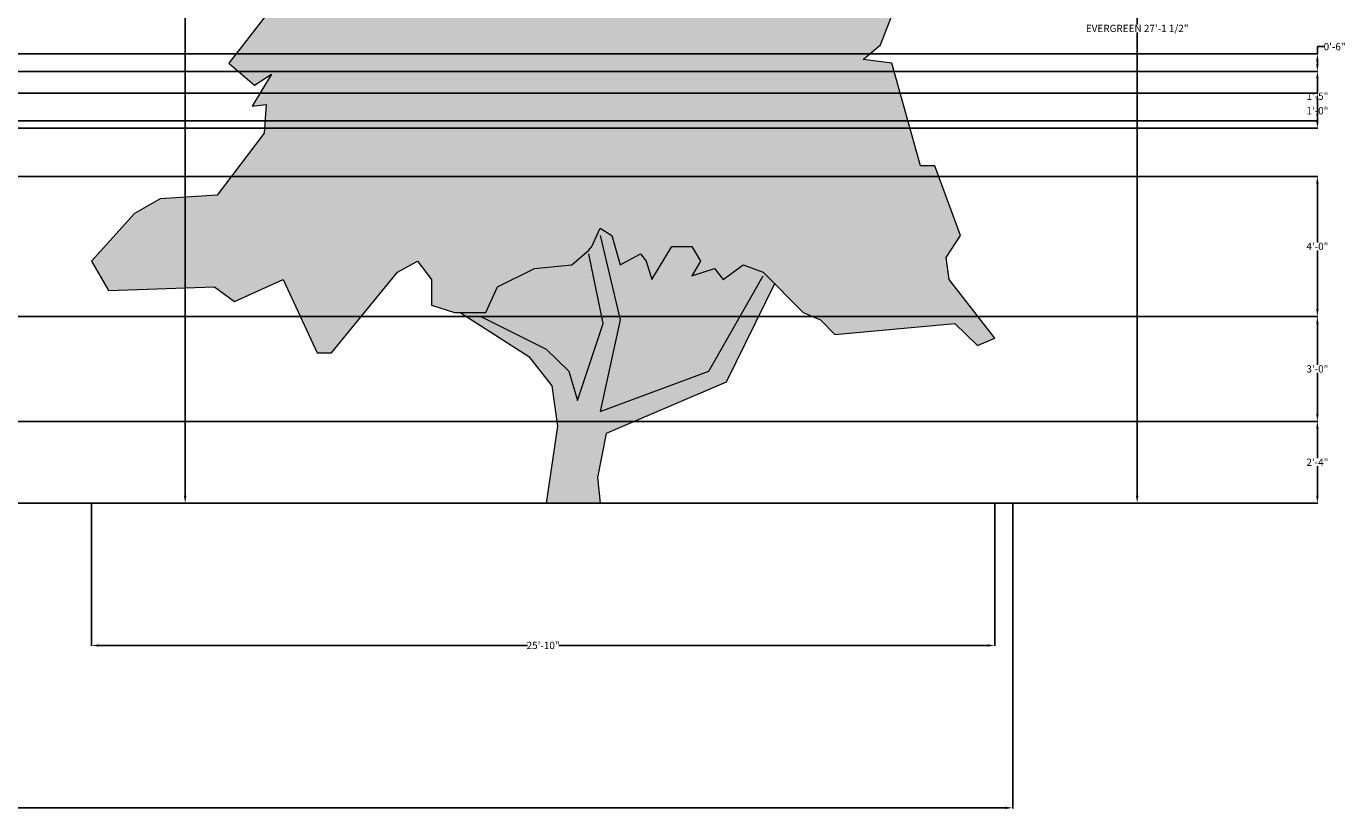
# Model space of a CAD drawing. Units: inches. Extents: x 481 to 2783, y 1975 to 3327.
# Tile 12 of 13: x 2331 to 2783, y 2017 to 2286. Entities that reach past the tile are written whole.
import ezdxf

# ---------------------------------------------------------------- set-up
doc = ezdxf.new("R2010")
doc.units = ezdxf.units.IN
doc.header["$MEASUREMENT"] = 0
for name, color, linetype, lineweight in [('A-ANNO-DIMS', 50, 'Continuous', 18), ('C-TOPO', 7, 'Continuous', 25), ('L-PLNT', 7, 'Continuous', 13)]:
    doc.layers.add(name, color=color, linetype=linetype, lineweight=lineweight)
doc.layers.add('L-PLNT-PATT', color=116, linetype='Continuous', lineweight=13, true_color=0x136734)
doc.layers.add('L-PLNT-TRNK-PATT', color=249, linetype='Continuous', lineweight=13, true_color=0x593132)
doc.styles.get("Standard").update_dxf_attribs({"font": 'arial.ttf'})
doc.dimstyles.get("Standard").update_dxf_attribs({"dimtxt": 2.5, "dimasz": 2.5, "dimexe": 0.18, "dimexo": 0.0625, "dimgap": 0.09, "dimtad": 0, "dimtih": 1, "dimtoh": 1, "dimzin": 0, "dimdsep": 46, "dimlunit": 3, "dimtxsty": 'Standard', "dimcen": 0.09, "dimadec": 0, "dimazin": 0, "dimtfac": 1, "dimtofl": 0, "dimtmove": 0, "dimatfit": 3, "dimfxl": 1, "dimtolj": 1, "dimtzin": 0, "dimarcsym": 0})

# ---------------------------------------------------------------- blocks, each defined once
blk = doc.blocks.new('Tree - type 3 evergreen elevation')
for points in [[(22.0124, 137.721), (18.5475, 141.5624), (15.5282, 138.2446), (13.8028, 139.3505), (13.3714, 142.1153), (11.2148, 143.2214), (8.1954, 140.4564), (4.7447, 141.0094), (2.1567, 136.0326), (2.1567, 131.6088), (5.6074, 129.9499), (3.0193, 128.2909), (0.4313, 130.5029), (-6.9015, 123.3141), (-6.9015, 121.6552), (-9.9208, 119.9963), (-9.0581, 118.3373), (-6.9015, 115.0195), (-10.7835, 112.2546), (-14.6656, 115.0195), (-16.8222, 114.4665), (-17.6849, 112.2546), (-14.6656, 111.7016), (-14.2342, 107.2778), (-17.6065, 107.8307), (-21.5669, 103.9599), (-17.2536, 103.4069), (-18.9789, 97.8771), (-22.8609, 97.3241), (-27.1743, 94.5593), (-32.3504, 91.7944), (-32.7817, 94.0063), (-36.6638, 85.7116), (-29.7624, 87.3705), (-25.449, 84.6056), (-26.743, 77.9699), (-34.507, 75.205), (-37.9578, 77.4169), (-39.2518, 74.099), (-42.2711, 73.5461), (-44.8592, 70.2282), (-47.8786, 66.3574), (-43.9965, 63.0395), (-41.4085, 64.6985), (-44.3346, 59.8898), (-42.2089, 60.1377), (-42.5159, 55.7849), (-49.6039, 46.4502), (-58.2307, 45.8972), (-62.1127, 43.6853), (-68.5828, 36.4966), (-65.9947, 32.0727), (-50.0352, 32.6257), (-47.0159, 30.4138), (-39.6831, 33.7317), (-34.507, 22.6721), (-32.3504, 22.6721), (-22.4296, 34.8376), (-19.4102, 36.4966), (-17.2536, 33.7317), (-17.2536, 29.8608), (-13.8028, 28.7549), (-9.0581, 28.7549), (-7.3328, 32.6257), (-1.7254, 35.3906), (3.8821, 35.9436), (6.4701, 38.1555), (6.9014, 38.7085), (8.1954, 41.4734), (9.9208, 40.3674), (11.2148, 35.9436), (14.2341, 37.6025), (15.0968, 36.4966), (15.9595, 33.7317), (18.9789, 38.7085), (21.9982, 38.7085), (23.2922, 36.4966), (21.9982, 34.2847), (25.4489, 35.3906), (26.743, 33.7317), (29.7623, 35.9436), (32.7817, 34.8376), (38.8204, 28.7549), (41.4084, 27.6489), (43.5651, 25.437), (61.6813, 27.0959), (65.132, 23.7781), (67.7201, 24.884), (60.8186, 33.7317), (60.3873, 37.0495), (62.544, 40.3674), (58.662, 50.874), (56.5053, 50.874), (52.1919, 66.3574), (47.8785, 66.9103), (50.4665, 69.1222), (53.9172, 77.9699), (47.0158, 85.1586), (38.3891, 87.9235), (42.2711, 94.0063)], [(42.2711, 94.0063), (38.8204, 104.5129), (36.6637, 104.5129), (32.3503, 113.9135), (29.7623, 113.3605), (26.743, 113.3605), (24.5862, 117.7844), (25.8802, 123.8671), (29.331, 123.8671), (22.8609, 131.6088), (21.9982, 137.6916)], [(8.1954, 40.3674), (11.2148, 27.6489), (8.1954, 13.8245), (24.5862, 19.9072), (32.7817, 34.2847)], [(-9.9208, 28.2019), (0, 23.2251), (3.4507, 19.9072), (4.7447, 15.4834), (8.6267, 27.0959), (6.4701, 37.6025)], [(34.5071, 33.1787), (27.1743, 18.2483), (9.0581, 10.5066), (7.7641, 3.8708), (8.1954, 0)], [(-12.9401, 28.7549), (-2.588, 22.1191), (0.8626, 17.6953), (1.7253, 11.6125), (0, 0)]]:
    blk.add_lwpolyline(points)
blk = doc.blocks.new('*D56')
at = {"layer": 'A-ANNO-DIMS', "color": 0, "lineweight": -2, "transparency": 16777216}
for p, q in [((2321.97, 2546.55), (2385.65, 2546.55)), ((2385.47, 2544.05), (2385.47, 2336.07)), ((2385.47, 2125.32), (2385.47, 2333.3)), ((2321.97, 2122.82), (2385.65, 2122.82))]:
    blk.add_line(p, q, dxfattribs=at)
at = {"layer": 'A-ANNO-DIMS', "color": 0, "transparency": 16777216}
for points in [[(2385.05, 2544.05), (2385.89, 2544.05), (2385.47, 2546.55)], [(2385.05, 2125.32), (2385.89, 2125.32), (2385.47, 2122.82)]]:
    blk.add_solid(points, dxfattribs=at)
at = {"layer": 'Defpoints', "color": 0, "transparency": 16777216}
for p in [(2321.91, 2546.55), (2385.47, 2546.55), (2321.91, 2122.82)]:
    blk.add_point(p, dxfattribs=at)
at = {"layer": 'A-ANNO-DIMS', "color": 0, "transparency": 16777216, "insert": (2385.47, 2334.69), "char_height": 2.5, "attachment_point": 5}
blk.add_mtext('\\A1;PALM 35\'-3 1/2"', dxfattribs=at)
blk = doc.blocks.new('*D60')
at = {"layer": 'A-ANNO-DIMS', "color": 0, "lineweight": -2, "transparency": 16777216}
for p, q in [((2663.19, 2448.32), (2712.14, 2448.32)), ((2711.96, 2445.82), (2711.96, 2286.95)), ((2711.96, 2125.32), (2711.96, 2284.19)), ((2663.19, 2122.82), (2712.14, 2122.82))]:
    blk.add_line(p, q, dxfattribs=at)
at = {"layer": 'A-ANNO-DIMS', "color": 0, "transparency": 16777216}
for points in [[(2711.54, 2445.82), (2712.37, 2445.82), (2711.96, 2448.32)], [(2711.54, 2125.32), (2712.37, 2125.32), (2711.96, 2122.82)]]:
    blk.add_solid(points, dxfattribs=at)
at = {"layer": 'Defpoints', "color": 0, "transparency": 16777216}
for p in [(2663.13, 2448.32), (2711.96, 2448.32), (2663.13, 2122.82)]:
    blk.add_point(p, dxfattribs=at)
at = {"layer": 'A-ANNO-DIMS', "color": 0, "transparency": 16777216, "insert": (2711.96, 2285.57), "char_height": 2.5, "attachment_point": 5}
blk.add_mtext('\\A1;EVERGREEN 27\'-1 1/2"', dxfattribs=at)
blk = doc.blocks.new('*D61')
at = {"layer": 'A-ANNO-DIMS', "color": 0, "lineweight": -2, "transparency": 16777216}
for p, q in [((2353.35, 2122.76), (2353.35, 2073.82)), ((2663.13, 2122.76), (2663.13, 2073.82)), ((2355.85, 2074), (2502.87, 2074)), ((2660.63, 2074), (2513.62, 2074))]:
    blk.add_line(p, q, dxfattribs=at)
at = {"layer": 'A-ANNO-DIMS', "color": 0, "transparency": 16777216}
for points in [[(2355.85, 2074.41), (2355.85, 2073.58), (2353.35, 2074)], [(2660.63, 2074.41), (2660.63, 2073.58), (2663.13, 2074)]]:
    blk.add_solid(points, dxfattribs=at)
at = {"layer": 'Defpoints', "color": 0, "transparency": 16777216}
for p in [(2353.35, 2122.82), (2663.13, 2122.82), (2663.13, 2074)]:
    blk.add_point(p, dxfattribs=at)
at = {"layer": 'A-ANNO-DIMS', "color": 0, "transparency": 16777216, "insert": (2508.24, 2074), "char_height": 2.5, "attachment_point": 5}
blk.add_mtext('\\A1;25\'-10"', dxfattribs=at)
blk = doc.blocks.new('*D66')
at = {"layer": 'A-ANNO-DIMS', "color": 0, "lineweight": -2, "transparency": 16777216}
for p, q in [((591.06, 2122.76), (591.06, 2018.14)), ((2669.26, 2122.76), (2669.26, 2018.14)), ((593.56, 2018.32), (1624.92, 2018.32)), ((2666.76, 2018.32), (1635.4, 2018.32))]:
    blk.add_line(p, q, dxfattribs=at)
at = {"layer": 'A-ANNO-DIMS', "color": 0, "transparency": 16777216}
for points in [[(593.56, 2018.74), (593.56, 2017.9), (591.06, 2018.32)], [(2666.76, 2018.74), (2666.76, 2017.9), (2669.26, 2018.32)]]:
    blk.add_solid(points, dxfattribs=at)
at = {"layer": 'Defpoints', "color": 0, "transparency": 16777216}
for p in [(591.06, 2122.82), (2669.26, 2122.82), (2669.26, 2018.32)]:
    blk.add_point(p, dxfattribs=at)
at = {"layer": 'A-ANNO-DIMS', "color": 0, "transparency": 16777216, "insert": (1630.16, 2018.32), "char_height": 2.5, "attachment_point": 5}
blk.add_mtext('\\A1;173\'-2"', dxfattribs=at)
blk = doc.blocks.new('*D70')
at = {"layer": 'A-ANNO-DIMS', "color": 0, "lineweight": -2, "transparency": 16777216}
for p, q in [((1794.5, 2150.82), (2773.94, 2150.82)), ((2773.76, 2148.32), (2773.76, 2138.17)), ((2773.76, 2125.32), (2773.76, 2135.48)), ((1794.5, 2122.82), (2773.94, 2122.82))]:
    blk.add_line(p, q, dxfattribs=at)
at = {"layer": 'A-ANNO-DIMS', "color": 0, "transparency": 16777216}
for points in [[(2773.34, 2148.32), (2774.17, 2148.32), (2773.76, 2150.82)], [(2773.34, 2125.32), (2774.17, 2125.32), (2773.76, 2122.82)]]:
    blk.add_solid(points, dxfattribs=at)
at = {"layer": 'Defpoints', "color": 0, "transparency": 16777216}
for p in [(1794.44, 2150.82), (2773.76, 2150.82), (1794.44, 2122.82)]:
    blk.add_point(p, dxfattribs=at)
at = {"layer": 'A-ANNO-DIMS', "color": 0, "transparency": 16777216, "insert": (2773.76, 2136.82), "char_height": 2.5, "attachment_point": 5}
blk.add_mtext('\\A1;2\'-4"', dxfattribs=at)
blk = doc.blocks.new('*D71')
at = {"layer": 'A-ANNO-DIMS', "color": 0, "lineweight": -2, "transparency": 16777216}
for p, q in [((1737.9, 2186.82), (2773.94, 2186.82)), ((2773.76, 2184.32), (2773.76, 2170.19)), ((2773.76, 2153.32), (2773.76, 2167.45)), ((1794.5, 2150.82), (2773.94, 2150.82))]:
    blk.add_line(p, q, dxfattribs=at)
at = {"layer": 'A-ANNO-DIMS', "color": 0, "transparency": 16777216}
for points in [[(2773.34, 2184.32), (2774.17, 2184.32), (2773.76, 2186.82)], [(2773.34, 2153.32), (2774.17, 2153.32), (2773.76, 2150.82)]]:
    blk.add_solid(points, dxfattribs=at)
at = {"layer": 'Defpoints', "color": 0, "transparency": 16777216}
for p in [(1737.84, 2186.82), (2773.76, 2186.82), (1794.44, 2150.82)]:
    blk.add_point(p, dxfattribs=at)
at = {"layer": 'A-ANNO-DIMS', "color": 0, "transparency": 16777216, "insert": (2773.76, 2168.82), "char_height": 2.5, "attachment_point": 5}
blk.add_mtext('\\A1;3\'-0"', dxfattribs=at)
blk = doc.blocks.new('*D72')
at = {"layer": 'A-ANNO-DIMS', "color": 0, "lineweight": -2, "transparency": 16777216}
for p, q in [((1737.9, 2234.82), (2773.94, 2234.82)), ((2773.76, 2232.32), (2773.76, 2212.19)), ((2773.76, 2189.32), (2773.76, 2209.45)), ((1737.9, 2186.82), (2773.94, 2186.82))]:
    blk.add_line(p, q, dxfattribs=at)
at = {"layer": 'A-ANNO-DIMS', "color": 0, "transparency": 16777216}
for points in [[(2773.34, 2232.32), (2774.17, 2232.32), (2773.76, 2234.82)], [(2773.34, 2189.32), (2774.17, 2189.32), (2773.76, 2186.82)]]:
    blk.add_solid(points, dxfattribs=at)
at = {"layer": 'Defpoints', "color": 0, "transparency": 16777216}
for p in [(1737.84, 2234.82), (2773.76, 2234.82), (1737.84, 2186.82)]:
    blk.add_point(p, dxfattribs=at)
at = {"layer": 'A-ANNO-DIMS', "color": 0, "transparency": 16777216, "insert": (2773.76, 2210.82), "char_height": 2.5, "attachment_point": 5}
blk.add_mtext('\\A1;4\'-0"', dxfattribs=at)
blk = doc.blocks.new('*D74')
at = {"layer": 'A-ANNO-DIMS', "color": 0, "lineweight": -2, "transparency": 16777216}
for p, q in [((1412.86, 2270.82), (2773.94, 2270.82)), ((2773.76, 2268.32), (2773.76, 2263.69)), ((2773.76, 2256.32), (2773.76, 2260.95)), ((1417, 2253.82), (2773.94, 2253.82))]:
    blk.add_line(p, q, dxfattribs=at)
at = {"layer": 'A-ANNO-DIMS', "color": 0, "transparency": 16777216}
for points in [[(2773.34, 2268.32), (2774.17, 2268.32), (2773.76, 2270.82)], [(2773.34, 2256.32), (2774.17, 2256.32), (2773.76, 2253.82)]]:
    blk.add_solid(points, dxfattribs=at)
at = {"layer": 'Defpoints', "color": 0, "transparency": 16777216}
for p in [(1412.79, 2270.82), (2773.76, 2270.82), (1416.94, 2253.82)]:
    blk.add_point(p, dxfattribs=at)
at = {"layer": 'A-ANNO-DIMS', "color": 0, "transparency": 16777216, "insert": (2773.76, 2262.32), "char_height": 2.5, "attachment_point": 5}
blk.add_mtext('\\A1;1\'-5"', dxfattribs=at)
blk = doc.blocks.new('*D75')
at = {"layer": 'A-ANNO-DIMS', "color": 0, "lineweight": -2, "transparency": 16777216}
for p, q in [((1794.5, 2276.82), (2773.94, 2276.82)), ((2773.76, 2276.82), (2773.76, 2279.32)), ((2773.76, 2279.32), (2776.26, 2279.32)), ((2773.76, 2273.32), (2773.76, 2274.32)), ((1794.5, 2270.82), (2773.94, 2270.82))]:
    blk.add_line(p, q, dxfattribs=at)
at = {"layer": 'A-ANNO-DIMS', "color": 0, "transparency": 16777216}
for points in [[(2773.34, 2274.32), (2774.17, 2274.32), (2773.76, 2276.82)], [(2773.34, 2273.32), (2774.17, 2273.32), (2773.76, 2270.82)]]:
    blk.add_solid(points, dxfattribs=at)
at = {"layer": 'Defpoints', "color": 0, "transparency": 16777216}
for p in [(1794.44, 2276.82), (2773.76, 2276.82), (1794.44, 2270.82)]:
    blk.add_point(p, dxfattribs=at)
at = {"layer": 'A-ANNO-DIMS', "color": 0, "transparency": 16777216, "insert": (2779.67, 2279.32), "char_height": 2.5, "attachment_point": 5}
blk.add_mtext('\\A1;0\'-6"', dxfattribs=at)
blk = doc.blocks.new('*D82')
at = {"layer": 'A-ANNO-DIMS', "color": 0, "lineweight": -2, "transparency": 16777216}
for p, q in [((1785.5, 2263.36), (2773.94, 2263.36)), ((2773.76, 2260.86), (2773.76, 2258.72)), ((2773.76, 2253.86), (2773.76, 2255.99)), ((1785.5, 2251.36), (2773.94, 2251.36))]:
    blk.add_line(p, q, dxfattribs=at)
at = {"layer": 'A-ANNO-DIMS', "color": 0, "transparency": 16777216}
for points in [[(2773.34, 2260.86), (2774.17, 2260.86), (2773.76, 2263.36)], [(2773.34, 2253.86), (2774.17, 2253.86), (2773.76, 2251.36)]]:
    blk.add_solid(points, dxfattribs=at)
at = {"layer": 'Defpoints', "color": 0, "transparency": 16777216}
for p in [(1785.44, 2263.36), (1785.44, 2251.36), (2773.76, 2251.36)]:
    blk.add_point(p, dxfattribs=at)
at = {"layer": 'A-ANNO-DIMS', "color": 0, "transparency": 16777216, "insert": (2773.76, 2257.36), "char_height": 2.5, "attachment_point": 5}
blk.add_mtext('\\A1;1\'-0"', dxfattribs=at)

msp = doc.modelspace()

# ---------------------------------------------------------------- hatches: boundary and pattern name
at = {"layer": 'L-PLNT-PATT'}
msp.add_hatch(color=256, dxfattribs=at).paths.add_polyline_path([(2476.873, 2366.633), (2469.209, 2367.89), (2460.208, 2359.093), (2470.011, 2357.836), (2466.089, 2345.268), (2457.267, 2344.011), (2447.464, 2337.728), (2435.7, 2331.444), (2434.72, 2336.471), (2425.897, 2317.619), (2441.582, 2321.389), (2451.385, 2315.106), (2448.444, 2300.025), (2430.798, 2293.741), (2422.956, 2298.768), (2420.015, 2291.227), (2413.153, 2289.97), (2407.271, 2282.43), (2400.408, 2273.633), (2409.231, 2266.092), (2415.113, 2269.862), (2408.463, 2258.933), (2413.294, 2259.497), (2412.596, 2249.604), (2396.487, 2228.389), (2376.881, 2227.132), (2368.058, 2222.105), (2353.354, 2205.767), (2359.236, 2195.713), (2395.507, 2196.97), (2402.369, 2191.943), (2419.035, 2199.483), (2430.798, 2174.348), (2435.7, 2174.348), (2458.247, 2201.997), (2465.109, 2205.767), (2470.011, 2199.483), (2470.011, 2190.686), (2477.853, 2188.172), (2488.637, 2188.172), (2492.558, 2196.97), (2505.302, 2203.254), (2518.046, 2204.51), (2523.928, 2209.537), (2524.908, 2210.794), (2527.849, 2217.078), (2531.77, 2214.564), (2534.711, 2204.51), (2541.573, 2208.281), (2543.534, 2205.767), (2545.495, 2199.483), (2552.357, 2210.794), (2559.219, 2210.794), (2562.16, 2205.767), (2559.219, 2200.74), (2567.062, 2203.254), (2570.003, 2199.483), (2576.865, 2204.51), (2583.727, 2201.997), (2597.451, 2188.172), (2603.333, 2185.659), (2608.235, 2180.632), (2649.408, 2184.402), (2657.25, 2176.862), (2663.132, 2179.375), (2647.447, 2199.483), (2646.467, 2207.024), (2651.368, 2214.564), (2642.546, 2238.443), (2637.644, 2238.443), (2627.841, 2273.633), (2618.038, 2274.889), (2623.92, 2279.916), (2631.762, 2300.025), (2616.077, 2316.362), (2596.471, 2322.646), (2605.294, 2336.471), (2597.451, 2360.349), (2592.55, 2360.349), (2582.746, 2381.714), (2576.865, 2380.458), (2570.003, 2380.458), (2565.101, 2390.512), (2568.042, 2404.336), (2575.884, 2404.336), (2561.18, 2421.931), (2559.202, 2435.877), (2551.377, 2444.553), (2544.515, 2437.012), (2540.593, 2439.526), (2539.613, 2445.809), (2534.711, 2448.323), (2527.849, 2442.039), (2520.007, 2443.296), (2514.125, 2431.985), (2514.125, 2421.931), (2521.967, 2418.161), (2516.085, 2414.39), (2510.203, 2419.417), (2493.538, 2403.079), (2493.538, 2399.309), (2486.676, 2395.539), (2488.637, 2391.768), (2493.538, 2384.228), (2484.715, 2377.944), (2475.892, 2384.228), (2470.991, 2382.971), (2469.03, 2377.944), (2475.892, 2376.687)])
at = {"layer": 'L-PLNT-TRNK-PATT'}
h = msp.add_hatch(color=256, dxfattribs=at)
h.paths.add_polyline_path([(2529.81, 2146.699), (2570.983, 2164.294), (2587.589, 2198.106), (2583.727, 2201.997), (2576.865, 2204.51), (2570.003, 2199.483), (2567.062, 2203.254), (2559.219, 2200.74), (2562.16, 2205.767), (2559.219, 2210.794), (2552.357, 2210.794), (2545.495, 2199.483), (2543.534, 2205.767), (2541.573, 2208.281), (2534.711, 2204.51), (2531.77, 2214.564), (2527.849, 2217.078), (2524.908, 2210.794), (2523.928, 2209.537), (2518.046, 2204.51), (2505.302, 2203.254), (2492.558, 2196.97), (2488.637, 2188.172), (2479.814, 2188.172), (2503.341, 2173.091), (2511.184, 2163.037), (2513.144, 2149.213), (2509.223, 2122.821), (2527.849, 2122.821), (2526.869, 2131.618)])
h.paths.add_polyline_path([(834.542, 2189.801), (831.106, 2193.262), (825, 2195.498), (818.895, 2191.026), (816.279, 2194.38), (809.302, 2192.144), (811.918, 2196.616), (809.302, 2201.089), (803.197, 2201.089), (797.091, 2191.026), (795.347, 2196.616), (793.603, 2198.852), (787.498, 2195.498), (784.881, 2204.443), (781.392, 2206.679), (778.776, 2201.089), (777.904, 2199.971), (772.671, 2195.498), (761.333, 2194.38), (749.995, 2188.789), (746.506, 2180.963), (738.657, 2180.963), (759.589, 2167.545), (766.566, 2158.6), (768.31, 2146.301), (764.821, 2122.821), (781.392, 2122.821), (780.52, 2130.647), (783.137, 2144.065), (819.768, 2159.718)])

# ---------------------------------------------------------------- linework, layer by layer
at = {"layer": 'C-TOPO'}
msp.add_line((1794.438, 2122.821), (2669.257, 2122.821), dxfattribs=at)

# ---------------------------------------------------------------- block references
at = {"layer": 'L-PLNT', "xscale": 2.272722171462171, "yscale": 2.272722171462171, "zscale": 2.272722171462171}
msp.add_blockref('Tree - type 3 evergreen elevation', (2509.223, 2122.821), dxfattribs=at)

# ---------------------------------------------------------------- dimensions: what is measured, and where the dimension line sits
at = {"layer": 'A-ANNO-DIMS'}
for base, p1, p2, text, picture, middle in [((2385.469, 2546.553), (2321.909, 2122.821), (2321.909, 2546.553), 'PALM <>', '*D56', (2385.469, 2334.687)), ((2711.958, 2448.323), (2663.132, 2122.821), (2663.132, 2448.323), 'EVERGREEN <>', '*D60', (2711.958, 2285.572))]:
    dim = msp.add_linear_dim(base=base, p1=p1, p2=p2, angle=90, text=text, dimstyle='Standard', override={"dimdec": 1, "dimlfac": 1, "dimrnd": 0, "dimzin": 1, "dimdsep": 46, "dimlunit": 4, "dimfrac": 2}, dxfattribs=at)
    dim.commit()
    dim.dimension.update_dxf_attribs({"geometry": picture, "text_midpoint": middle})
for base, p1, p2, picture, middle in [((2773.757, 2276.821), (1794.438, 2270.821), (1794.438, 2276.821), '*D75', (2779.67, 2279.321)), ((2773.757, 2270.821), (1416.938, 2253.821), (1412.793, 2270.821), '*D74', (2773.757, 2262.321)), ((2773.757, 2251.356), (1785.438, 2263.356), (1785.438, 2251.356), '*D82', (2773.757, 2257.356)), ((2773.757, 2234.821), (1737.842, 2186.821), (1737.842, 2234.821), '*D72', (2773.757, 2210.821)), ((2773.757, 2186.821), (1794.438, 2150.821), (1737.842, 2186.821), '*D71', (2773.757, 2168.821)), ((2773.757, 2150.821), (1794.438, 2122.821), (1794.438, 2150.821), '*D70', (2773.757, 2136.821))]:
    dim = msp.add_linear_dim(base=base, p1=p1, p2=p2, angle=90, dimstyle='Standard', override={"dimdec": 1, "dimlfac": 1, "dimrnd": 0, "dimzin": 1, "dimdsep": 46, "dimlunit": 4, "dimfrac": 2}, dxfattribs=at)
    dim.commit()
    dim.dimension.update_dxf_attribs({"geometry": picture, "text_midpoint": middle})
for base, p1, p2, picture, middle in [((2669.257, 2018.321), (591.063, 2122.821), (2669.257, 2122.821), '*D66', (1630.16, 2018.321)), ((2663.132, 2073.995), (2353.354, 2122.821), (2663.132, 2122.821), '*D61', (2508.243, 2073.995))]:
    dim = msp.add_linear_dim(base=base, p1=p1, p2=p2, dimstyle='Standard', override={"dimdec": 1, "dimlfac": 1, "dimrnd": 0, "dimzin": 1, "dimdsep": 46, "dimlunit": 4, "dimfrac": 2}, dxfattribs=at)
    dim.commit()
    dim.dimension.update_dxf_attribs({"geometry": picture, "text_midpoint": middle})

doc.saveas('drawing.dxf')
